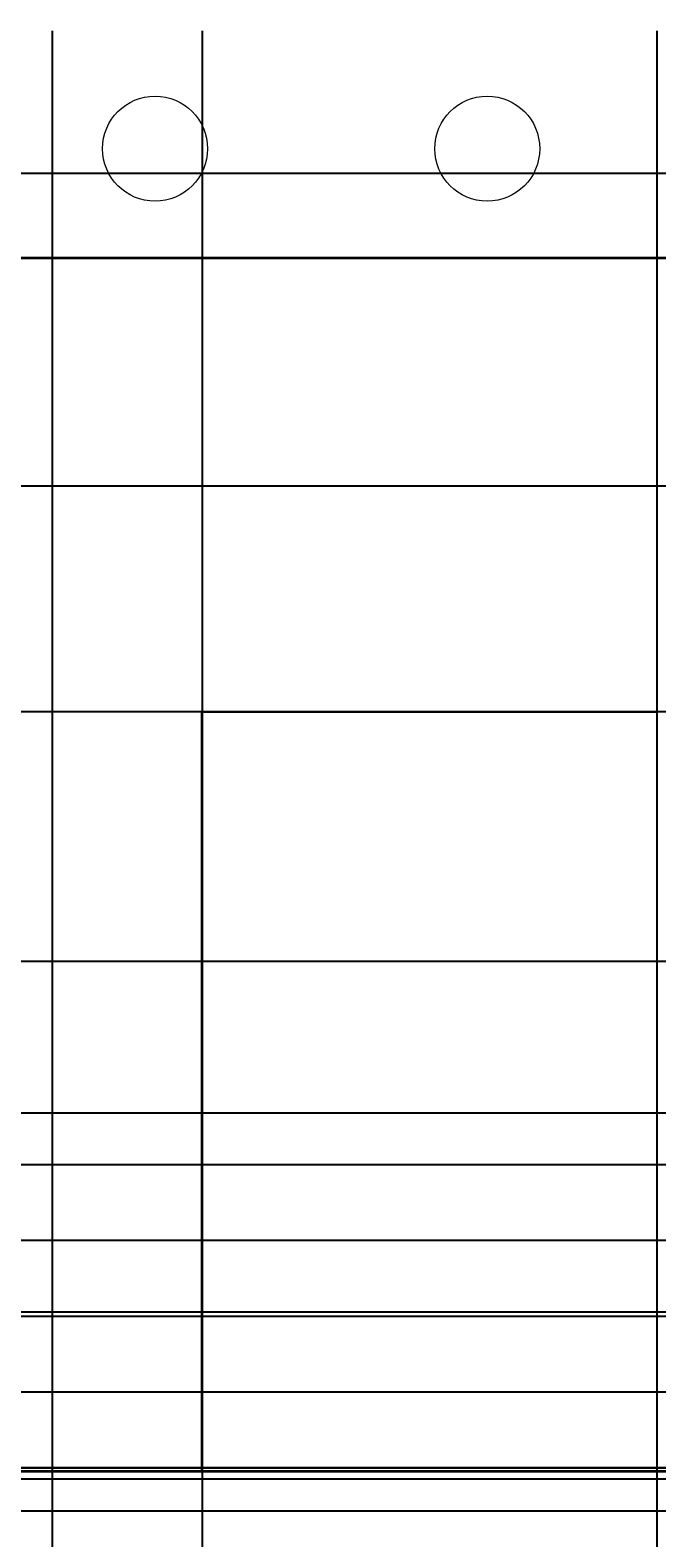
# Model space of a CAD drawing. Units: inches. Extents: x -13 to 809, y 112 to 656.
# Tile 9 of 55: x 111 to 161, y 205 to 325. Entities that reach past the tile are written whole.
import ezdxf

# ---------------------------------------------------------------- set-up
doc = ezdxf.new("R2010")
doc.units = ezdxf.units.IN
doc.header["$MEASUREMENT"] = 0
for name, color, linetype, lineweight in [('A-ANNO-DIMS', 2, 'Continuous', 18), ('A-DOOR', 4, 'Continuous', 25), ('A-ELEV', 7, 'Continuous', 35), ('A-ELEV-OTLN', 7, 'Continuous', 18)]:
    doc.layers.add(name, color=color, linetype=linetype, lineweight=lineweight)
doc.styles.get("Standard").update_dxf_attribs({"font": 'arial.ttf'})
doc.dimstyles.get("Standard").update_dxf_attribs({"dimtxt": 0.625, "dimasz": 0.18, "dimexe": 0.18, "dimexo": 0.0625, "dimgap": 0.09, "dimtad": 0, "dimtih": 1, "dimtoh": 1, "dimdec": 4, "dimzin": 0, "dimdsep": 46, "dimlunit": 4, "dimtxsty": 'Standard', "dimcen": 0.09, "dimadec": 0, "dimazin": 0, "dimtfac": 1, "dimtdec": 4, "dimtofl": 0, "dimtmove": 0, "dimatfit": 3, "dimfxl": 1, "dimtolj": 1, "dimtzin": 0, "dimarcsym": 0})

# ---------------------------------------------------------------- blocks, each defined once
blk = doc.blocks.new('*D12')
at = {"layer": 'A-ANNO-DIMS', "color": 0, "lineweight": -2, "transparency": 16777216}
for p, q in [((95.05, 306.46), (95.05, 112.34)), ((124.92, 210.46), (124.92, 112.34)), ((95.23, 112.52), (108.83, 112.52)), ((124.74, 112.52), (111.13, 112.52))]:
    blk.add_line(p, q, dxfattribs=at)
at = {"layer": 'A-ANNO-DIMS', "color": 0, "transparency": 16777216}
for points in [[(95.23, 112.55), (95.23, 112.49), (95.05, 112.52)], [(124.74, 112.55), (124.74, 112.49), (124.92, 112.52)]]:
    blk.add_solid(points, dxfattribs=at)
at = {"layer": 'Defpoints', "color": 0, "transparency": 16777216}
for p in [(95.05, 306.52), (124.92, 210.52), (124.92, 112.52)]:
    blk.add_point(p, dxfattribs=at)
at = {"layer": 'A-ANNO-DIMS', "color": 0, "transparency": 16777216, "insert": (109.98, 112.52), "char_height": 0.625, "attachment_point": 5}
blk.add_mtext('\\A1;29.87', dxfattribs=at)
blk = doc.blocks.new('*D13')
at = {"layer": 'A-ANNO-DIMS', "color": 0, "lineweight": -2, "transparency": 16777216}
for p, q in [((124.92, 210.46), (124.92, 112.34)), ((160.92, 210.46), (160.92, 112.34)), ((125.1, 112.52), (142.38, 112.52)), ((160.74, 112.52), (143.46, 112.52))]:
    blk.add_line(p, q, dxfattribs=at)
at = {"layer": 'A-ANNO-DIMS', "color": 0, "transparency": 16777216}
for points in [[(125.1, 112.55), (125.1, 112.49), (124.92, 112.52)], [(160.74, 112.55), (160.74, 112.49), (160.92, 112.52)]]:
    blk.add_solid(points, dxfattribs=at)
at = {"layer": 'Defpoints', "color": 0, "transparency": 16777216}
for p in [(124.92, 210.52), (160.92, 210.52), (160.92, 112.52)]:
    blk.add_point(p, dxfattribs=at)
at = {"layer": 'A-ANNO-DIMS', "color": 0, "transparency": 16777216, "insert": (142.92, 112.52), "char_height": 0.625, "attachment_point": 5}
blk.add_mtext('\\A1;36', dxfattribs=at)
blk = doc.blocks.new('*D39')
at = {"layer": 'A-ANNO-DIMS', "color": 0, "lineweight": -2, "transparency": 16777216}
for p, q in [((341.34, 524.28), (-12.1, 524.28)), ((-11.92, 524.1), (-11.92, 406.78)), ((-11.92, 288.63), (-11.92, 405.96)), ((341.34, 288.45), (-12.1, 288.45))]:
    blk.add_line(p, q, dxfattribs=at)
at = {"layer": 'A-ANNO-DIMS', "color": 0, "transparency": 16777216}
for points in [[(-11.95, 524.1), (-11.89, 524.1), (-11.92, 524.28)], [(-11.95, 288.63), (-11.89, 288.63), (-11.92, 288.45)]]:
    blk.add_solid(points, dxfattribs=at)
at = {"layer": 'Defpoints', "color": 0, "transparency": 16777216}
for p in [(-11.92, 524.28), (341.41, 524.28), (341.41, 288.45)]:
    blk.add_point(p, dxfattribs=at)
at = {"layer": 'A-ANNO-DIMS', "color": 0, "transparency": 16777216, "insert": (-11.92, 406.37), "char_height": 0.625, "attachment_point": 5}
blk.add_mtext('\\A1;235.83', dxfattribs=at)
blk = doc.blocks.new('*D40')
at = {"layer": 'A-ANNO-DIMS', "color": 0, "lineweight": -2, "transparency": 16777216}
for p, q in [((471.04, 313.17), (-12.1, 313.17)), ((-11.92, 312.99), (-11.92, 301.22)), ((-11.92, 288.63), (-11.92, 300.4)), ((341.34, 288.45), (-12.1, 288.45))]:
    blk.add_line(p, q, dxfattribs=at)
at = {"layer": 'A-ANNO-DIMS', "color": 0, "transparency": 16777216}
for points in [[(-11.95, 312.99), (-11.89, 312.99), (-11.92, 313.17)], [(-11.95, 288.63), (-11.89, 288.63), (-11.92, 288.45)]]:
    blk.add_solid(points, dxfattribs=at)
at = {"layer": 'Defpoints', "color": 0, "transparency": 16777216}
for p in [(471.1, 313.17), (-11.92, 288.45), (341.41, 288.45)]:
    blk.add_point(p, dxfattribs=at)
at = {"layer": 'A-ANNO-DIMS', "color": 0, "transparency": 16777216, "insert": (-11.92, 300.81), "char_height": 0.625, "attachment_point": 5}
blk.add_mtext('\\A1;24.716', dxfattribs=at)
blk = doc.blocks.new('*D41')
at = {"layer": 'A-ANNO-DIMS', "color": 0, "lineweight": -2, "transparency": 16777216}
for p, q in [((471.04, 357.98), (-12.1, 357.98)), ((-11.92, 357.8), (-11.92, 335.98)), ((-11.92, 313.35), (-11.92, 335.16)), ((471.04, 313.17), (-12.1, 313.17))]:
    blk.add_line(p, q, dxfattribs=at)
at = {"layer": 'A-ANNO-DIMS', "color": 0, "transparency": 16777216}
for points in [[(-11.95, 357.8), (-11.89, 357.8), (-11.92, 357.98)], [(-11.95, 313.35), (-11.89, 313.35), (-11.92, 313.17)]]:
    blk.add_solid(points, dxfattribs=at)
at = {"layer": 'Defpoints', "color": 0, "transparency": 16777216}
for p in [(-11.92, 357.98), (471.1, 357.98), (471.1, 313.17)]:
    blk.add_point(p, dxfattribs=at)
at = {"layer": 'A-ANNO-DIMS', "color": 0, "transparency": 16777216, "insert": (-11.92, 335.57), "char_height": 0.625, "attachment_point": 5}
blk.add_mtext('\\A1;44.81', dxfattribs=at)
blk = doc.blocks.new('*D44')
at = {"layer": 'A-ANNO-DIMS', "color": 0, "lineweight": -2, "transparency": 16777216}
for p, q in [((124.86, 270.6), (-12.1, 270.6)), ((-11.92, 270.42), (-11.92, 240.97)), ((-11.92, 210.7), (-11.92, 240.15)), ((124.86, 210.52), (-12.1, 210.52))]:
    blk.add_line(p, q, dxfattribs=at)
at = {"layer": 'A-ANNO-DIMS', "color": 0, "transparency": 16777216}
for points in [[(-11.95, 270.42), (-11.89, 270.42), (-11.92, 270.6)], [(-11.95, 210.7), (-11.89, 210.7), (-11.92, 210.52)]]:
    blk.add_solid(points, dxfattribs=at)
at = {"layer": 'Defpoints', "color": 0, "transparency": 16777216}
for p in [(-11.92, 270.6), (124.92, 270.6), (124.92, 210.52)]:
    blk.add_point(p, dxfattribs=at)
at = {"layer": 'A-ANNO-DIMS', "color": 0, "transparency": 16777216, "insert": (-11.92, 240.56), "char_height": 0.625, "attachment_point": 5}
blk.add_mtext('\\A1;60.08', dxfattribs=at)
blk = doc.blocks.new('*D45')
at = {"layer": 'A-ANNO-DIMS', "color": 0, "lineweight": -2, "transparency": 16777216}
for p, q in [((275.65, 270.6), (-12.1, 270.6)), ((-11.92, 270.42), (-11.92, 247.26)), ((-11.92, 223.28), (-11.92, 246.44)), ((275.65, 223.1), (-12.1, 223.1))]:
    blk.add_line(p, q, dxfattribs=at)
at = {"layer": 'A-ANNO-DIMS', "color": 0, "transparency": 16777216}
for points in [[(-11.95, 270.42), (-11.89, 270.42), (-11.92, 270.6)], [(-11.95, 223.28), (-11.89, 223.28), (-11.92, 223.1)]]:
    blk.add_solid(points, dxfattribs=at)
at = {"layer": 'Defpoints', "color": 0, "transparency": 16777216}
for p in [(-11.92, 270.6), (275.71, 270.6), (275.71, 223.1)]:
    blk.add_point(p, dxfattribs=at)
at = {"layer": 'A-ANNO-DIMS', "color": 0, "transparency": 16777216, "insert": (-11.92, 246.85), "char_height": 0.625, "attachment_point": 5}
blk.add_mtext('\\A1;47.5', dxfattribs=at)
blk = doc.blocks.new('*D49')
at = {"layer": 'A-ANNO-DIMS', "color": 0, "lineweight": -2, "transparency": 16777216}
for p, q in [((590.95, 250.84), (-12.1, 250.84)), ((-11.92, 250.66), (-11.92, 245.25)), ((-11.92, 239.02), (-11.92, 244.44)), ((590.95, 238.84), (-12.1, 238.84))]:
    blk.add_line(p, q, dxfattribs=at)
at = {"layer": 'A-ANNO-DIMS', "color": 0, "transparency": 16777216}
for points in [[(-11.95, 250.66), (-11.89, 250.66), (-11.92, 250.84)], [(-11.95, 239.02), (-11.89, 239.02), (-11.92, 238.84)]]:
    blk.add_solid(points, dxfattribs=at)
at = {"layer": 'Defpoints', "color": 0, "transparency": 16777216}
for p in [(-11.92, 250.84), (591.01, 250.84), (591.01, 238.84)]:
    blk.add_point(p, dxfattribs=at)
at = {"layer": 'A-ANNO-DIMS', "color": 0, "transparency": 16777216, "insert": (-11.92, 244.84), "char_height": 0.625, "attachment_point": 5}
blk.add_mtext('\\A1;12', dxfattribs=at)
blk = doc.blocks.new('*D50')
at = {"layer": 'A-ANNO-DIMS', "color": 0, "lineweight": -2, "transparency": 16777216}
for p, q in [((590.95, 238.84), (-12.1, 238.84)), ((-11.92, 238.66), (-11.92, 224.77)), ((-11.92, 210.06), (-11.92, 223.95)), ((607.51, 209.88), (-12.1, 209.88))]:
    blk.add_line(p, q, dxfattribs=at)
at = {"layer": 'A-ANNO-DIMS', "color": 0, "transparency": 16777216}
for points in [[(-11.95, 238.66), (-11.89, 238.66), (-11.92, 238.84)], [(-11.95, 210.06), (-11.89, 210.06), (-11.92, 209.88)]]:
    blk.add_solid(points, dxfattribs=at)
at = {"layer": 'Defpoints', "color": 0, "transparency": 16777216}
for p in [(591.01, 238.84), (-11.92, 209.88), (607.57, 209.88)]:
    blk.add_point(p, dxfattribs=at)
at = {"layer": 'A-ANNO-DIMS', "color": 0, "transparency": 16777216, "insert": (-11.92, 224.36), "char_height": 0.625, "attachment_point": 5}
blk.add_mtext('\\A1;28.97', dxfattribs=at)
blk = doc.blocks.new('*D80')
at = {"layer": 'A-ANNO-DIMS', "color": 0, "lineweight": -2, "transparency": 16777216}
for p, q in [((368.83, 216.77), (-12.1, 216.77)), ((-11.92, 216.59), (-11.92, 214.18)), ((-11.92, 210.95), (-11.92, 213.36)), ((368.83, 210.77), (-12.1, 210.77))]:
    blk.add_line(p, q, dxfattribs=at)
at = {"layer": 'A-ANNO-DIMS', "color": 0, "transparency": 16777216}
for points in [[(-11.95, 216.59), (-11.89, 216.59), (-11.92, 216.77)], [(-11.95, 210.95), (-11.89, 210.95), (-11.92, 210.77)]]:
    blk.add_solid(points, dxfattribs=at)
at = {"layer": 'Defpoints', "color": 0, "transparency": 16777216}
for p in [(-11.92, 216.77), (368.9, 216.77), (368.9, 210.77)]:
    blk.add_point(p, dxfattribs=at)
at = {"layer": 'A-ANNO-DIMS', "color": 0, "transparency": 16777216, "insert": (-11.92, 213.77), "char_height": 0.625, "attachment_point": 5}
blk.add_mtext('\\A1;6', dxfattribs=at)
blk = doc.blocks.new('*D81')
at = {"layer": 'A-ANNO-DIMS', "color": 0, "lineweight": -2, "transparency": 16777216}
for p, q in [((378.83, 222.77), (-12.1, 222.77)), ((-11.92, 222.59), (-11.92, 220.18)), ((-11.92, 216.95), (-11.92, 219.36)), ((378.83, 216.77), (-12.1, 216.77))]:
    blk.add_line(p, q, dxfattribs=at)
at = {"layer": 'A-ANNO-DIMS', "color": 0, "transparency": 16777216}
for points in [[(-11.95, 222.59), (-11.89, 222.59), (-11.92, 222.77)], [(-11.95, 216.95), (-11.89, 216.95), (-11.92, 216.77)]]:
    blk.add_solid(points, dxfattribs=at)
at = {"layer": 'Defpoints', "color": 0, "transparency": 16777216}
for p in [(-11.92, 222.77), (378.9, 222.77), (378.9, 216.77)]:
    blk.add_point(p, dxfattribs=at)
at = {"layer": 'A-ANNO-DIMS', "color": 0, "transparency": 16777216, "insert": (-11.92, 219.77), "char_height": 0.625, "attachment_point": 5}
blk.add_mtext('\\A1;6', dxfattribs=at)
blk = doc.blocks.new('*D82')
at = {"layer": 'A-ANNO-DIMS', "color": 0, "lineweight": -2, "transparency": 16777216}
for p, q in [((388.83, 228.77), (-12.1, 228.77)), ((-11.92, 228.59), (-11.92, 226.18)), ((-11.92, 222.95), (-11.92, 225.36)), ((388.83, 222.77), (-12.1, 222.77))]:
    blk.add_line(p, q, dxfattribs=at)
at = {"layer": 'A-ANNO-DIMS', "color": 0, "transparency": 16777216}
for points in [[(-11.95, 228.59), (-11.89, 228.59), (-11.92, 228.77)], [(-11.95, 222.95), (-11.89, 222.95), (-11.92, 222.77)]]:
    blk.add_solid(points, dxfattribs=at)
at = {"layer": 'Defpoints', "color": 0, "transparency": 16777216}
for p in [(-11.92, 228.77), (388.9, 228.77), (388.9, 222.77)]:
    blk.add_point(p, dxfattribs=at)
at = {"layer": 'A-ANNO-DIMS', "color": 0, "transparency": 16777216, "insert": (-11.92, 225.77), "char_height": 0.625, "attachment_point": 5}
blk.add_mtext('\\A1;6', dxfattribs=at)
blk = doc.blocks.new('*D83')
at = {"layer": 'A-ANNO-DIMS', "color": 0, "lineweight": -2, "transparency": 16777216}
for p, q in [((398.83, 234.77), (-12.1, 234.77)), ((-11.92, 234.59), (-11.92, 232.18)), ((-11.92, 228.95), (-11.92, 231.36)), ((398.83, 228.77), (-12.1, 228.77))]:
    blk.add_line(p, q, dxfattribs=at)
at = {"layer": 'A-ANNO-DIMS', "color": 0, "transparency": 16777216}
for points in [[(-11.95, 234.59), (-11.89, 234.59), (-11.92, 234.77)], [(-11.95, 228.95), (-11.89, 228.95), (-11.92, 228.77)]]:
    blk.add_solid(points, dxfattribs=at)
at = {"layer": 'Defpoints', "color": 0, "transparency": 16777216}
for p in [(-11.92, 234.77), (398.9, 234.77), (398.9, 228.77)]:
    blk.add_point(p, dxfattribs=at)
at = {"layer": 'A-ANNO-DIMS', "color": 0, "transparency": 16777216, "insert": (-11.92, 231.77), "char_height": 0.625, "attachment_point": 5}
blk.add_mtext('\\A1;6', dxfattribs=at)
blk = doc.blocks.new('*D84')
at = {"layer": 'A-ANNO-DIMS', "color": 0, "lineweight": -2, "transparency": 16777216}
for p, q in [((408.83, 238.84), (-12.1, 238.84)), ((-11.92, 238.66), (-11.92, 237.22)), ((-11.92, 234.95), (-11.92, 236.4)), ((408.83, 234.77), (-12.1, 234.77))]:
    blk.add_line(p, q, dxfattribs=at)
at = {"layer": 'A-ANNO-DIMS', "color": 0, "transparency": 16777216}
for points in [[(-11.95, 238.66), (-11.89, 238.66), (-11.92, 238.84)], [(-11.95, 234.95), (-11.89, 234.95), (-11.92, 234.77)]]:
    blk.add_solid(points, dxfattribs=at)
at = {"layer": 'Defpoints', "color": 0, "transparency": 16777216}
for p in [(-11.92, 238.84), (408.9, 238.84), (408.9, 234.77)]:
    blk.add_point(p, dxfattribs=at)
at = {"layer": 'A-ANNO-DIMS', "color": 0, "transparency": 16777216, "insert": (-11.92, 236.81), "char_height": 0.625, "attachment_point": 5}
blk.add_mtext('\\A1;4.069', dxfattribs=at)
blk = doc.blocks.new('*D94')
at = {"layer": 'A-ANNO-DIMS', "color": 0, "lineweight": -2, "transparency": 16777216}
for p, q in [((210.02, 223.1), (-12.1, 223.1)), ((-11.92, 222.92), (-11.92, 217.22)), ((-11.92, 210.7), (-11.92, 216.4)), ((160.86, 210.52), (-12.1, 210.52))]:
    blk.add_line(p, q, dxfattribs=at)
at = {"layer": 'A-ANNO-DIMS', "color": 0, "transparency": 16777216}
for points in [[(-11.95, 222.92), (-11.89, 222.92), (-11.92, 223.1)], [(-11.95, 210.7), (-11.89, 210.7), (-11.92, 210.52)]]:
    blk.add_solid(points, dxfattribs=at)
at = {"layer": 'Defpoints', "color": 0, "transparency": 16777216}
for p in [(-11.92, 223.1), (210.08, 223.1), (160.92, 210.52)]:
    blk.add_point(p, dxfattribs=at)
at = {"layer": 'A-ANNO-DIMS', "color": 0, "transparency": 16777216, "insert": (-11.92, 216.81), "char_height": 0.625, "attachment_point": 5}
blk.add_mtext('\\A1;12.58', dxfattribs=at)
blk = doc.blocks.new('*D107')
at = {"layer": 'A-ANNO-DIMS', "color": 0, "lineweight": -2, "transparency": 16777216}
for p, q in [((113.05, 324.46), (113.05, 112.34)), ((95.05, 306.46), (95.05, 112.34)), ((95.23, 112.52), (102.93, 112.52)), ((112.87, 112.52), (105.16, 112.52))]:
    blk.add_line(p, q, dxfattribs=at)
at = {"layer": 'A-ANNO-DIMS', "color": 0, "transparency": 16777216}
for points in [[(95.23, 112.55), (95.23, 112.49), (95.05, 112.52)], [(112.87, 112.55), (112.87, 112.49), (113.05, 112.52)]]:
    blk.add_solid(points, dxfattribs=at)
at = {"layer": 'Defpoints', "color": 0, "transparency": 16777216}
for p in [(113.05, 324.52), (95.05, 306.52), (113.05, 112.52)]:
    blk.add_point(p, dxfattribs=at)
at = {"layer": 'A-ANNO-DIMS', "color": 0, "transparency": 16777216, "insert": (104.05, 112.52), "char_height": 0.625, "attachment_point": 5}
blk.add_mtext('\\A1;18.00', dxfattribs=at)
blk = doc.blocks.new('*D109')
at = {"layer": 'A-ANNO-DIMS', "color": 0, "lineweight": -2, "transparency": 16777216}
for p, q in [((113.05, 324.46), (113.05, 112.34)), ((124.92, 324.46), (124.92, 112.34)), ((113.23, 112.52), (117.63, 112.52)), ((124.74, 112.52), (120.34, 112.52))]:
    blk.add_line(p, q, dxfattribs=at)
at = {"layer": 'A-ANNO-DIMS', "color": 0, "transparency": 16777216}
for points in [[(113.23, 112.55), (113.23, 112.49), (113.05, 112.52)], [(124.74, 112.55), (124.74, 112.49), (124.92, 112.52)]]:
    blk.add_solid(points, dxfattribs=at)
at = {"layer": 'Defpoints', "color": 0, "transparency": 16777216}
for p in [(113.05, 324.52), (124.92, 324.52), (124.92, 112.52)]:
    blk.add_point(p, dxfattribs=at)
at = {"layer": 'A-ANNO-DIMS', "color": 0, "transparency": 16777216, "insert": (118.98, 112.52), "char_height": 0.625, "attachment_point": 5}
blk.add_mtext('\\A1;11.872', dxfattribs=at)
blk = doc.blocks.new('*D110')
at = {"layer": 'A-ANNO-DIMS', "color": 0, "lineweight": -2, "transparency": 16777216}
for p, q in [((124.92, 324.46), (124.92, 112.34)), ((160.92, 324.46), (160.92, 112.34)), ((125.1, 112.52), (141.78, 112.52)), ((160.74, 112.52), (144.06, 112.52))]:
    blk.add_line(p, q, dxfattribs=at)
at = {"layer": 'A-ANNO-DIMS', "color": 0, "transparency": 16777216}
for points in [[(125.1, 112.55), (125.1, 112.49), (124.92, 112.52)], [(160.74, 112.55), (160.74, 112.49), (160.92, 112.52)]]:
    blk.add_solid(points, dxfattribs=at)
at = {"layer": 'Defpoints', "color": 0, "transparency": 16777216}
for p in [(124.92, 324.52), (160.92, 324.52), (160.92, 112.52)]:
    blk.add_point(p, dxfattribs=at)
at = {"layer": 'A-ANNO-DIMS', "color": 0, "transparency": 16777216, "insert": (142.92, 112.52), "char_height": 0.625, "attachment_point": 5}
blk.add_mtext('\\A1;36.00', dxfattribs=at)
blk = doc.blocks.new('*D115')
at = {"layer": 'A-ANNO-DIMS', "color": 0, "lineweight": -2, "transparency": 16777216}
for p, q in [((311.4, 210.78), (-12.1, 210.78)), ((-11.92, 210.6), (-11.92, 181.06)), ((-11.92, 150.7), (-11.92, 180.24)), ((311.64, 150.52), (-12.1, 150.52))]:
    blk.add_line(p, q, dxfattribs=at)
at = {"layer": 'A-ANNO-DIMS', "color": 0, "transparency": 16777216}
for points in [[(-11.95, 210.6), (-11.89, 210.6), (-11.92, 210.78)], [(-11.95, 150.7), (-11.89, 150.7), (-11.92, 150.52)]]:
    blk.add_solid(points, dxfattribs=at)
at = {"layer": 'Defpoints', "color": 0, "transparency": 16777216}
for p in [(-11.92, 210.78), (311.46, 210.78), (311.7, 150.52)]:
    blk.add_point(p, dxfattribs=at)
at = {"layer": 'A-ANNO-DIMS', "color": 0, "transparency": 16777216, "insert": (-11.92, 180.65), "char_height": 0.625, "attachment_point": 5}
blk.add_mtext('\\A1;60.27', dxfattribs=at)
blk = doc.blocks.new('*D118')
at = {"layer": 'A-ANNO-DIMS', "color": 0, "lineweight": -2, "transparency": 16777216}
for p, q in [((311.4, 210.78), (-12.1, 210.78)), ((-11.92, 210.6), (-11.92, 209.49)), ((-11.92, 207.55), (-11.92, 208.67)), ((308.59, 207.37), (-12.1, 207.37))]:
    blk.add_line(p, q, dxfattribs=at)
at = {"layer": 'A-ANNO-DIMS', "color": 0, "transparency": 16777216}
for points in [[(-11.95, 210.6), (-11.89, 210.6), (-11.92, 210.78)], [(-11.95, 207.55), (-11.89, 207.55), (-11.92, 207.37)]]:
    blk.add_solid(points, dxfattribs=at)
at = {"layer": 'Defpoints', "color": 0, "transparency": 16777216}
for p in [(-11.92, 210.78), (311.46, 210.78), (308.65, 207.37)]:
    blk.add_point(p, dxfattribs=at)
at = {"layer": 'A-ANNO-DIMS', "color": 0, "transparency": 16777216, "insert": (-11.92, 209.08), "char_height": 0.625, "attachment_point": 5}
blk.add_mtext('\\A1;3.41', dxfattribs=at)

msp = doc.modelspace()

# ---------------------------------------------------------------- linework, layer by layer
at = {"layer": 'A-DOOR'}
for p, q in [((124.9184, 210.5199), (124.9184, 270.6024)), ((124.9184, 270.6024), (160.9184, 270.6024)), ((160.9184, 270.6024), (160.9184, 210.5199))]:
    msp.add_line(p, q, dxfattribs=at)
at = {"layer": 'A-ELEV'}
for p, q in [((109.5888, 306.5199), (337.5074, 306.5199)), ((26.0809, 210.5199), (256.4464, 210.5199))]:
    msp.add_line(p, q, dxfattribs=at)
at = {"layer": 'A-ELEV-OTLN'}
for centre in [(121.2048, 315.1435), (147.4935, 315.1435)]:
    msp.add_circle(centre, 4.1542, dxfattribs=at)

# ---------------------------------------------------------------- dimensions: what is measured, and where the dimension line sits
at = {"layer": 'A-ANNO-DIMS'}
for base, p1, p2, override, picture, middle in [((-11.9191, 524.281), (341.4072, 288.4508), (341.4072, 524.281), {"dimdec": 2, "dimlfac": 1, "dimrnd": 0, "dimzin": 0, "dimdsep": 46, "dimlunit": 2}, '*D39', (-11.9191, 406.3659)), ((-11.9191, 357.9804), (471.0998, 313.1667), (471.0998, 357.9804), {"dimdec": 2, "dimlfac": 1, "dimrnd": 0, "dimzin": 0, "dimdsep": 46, "dimlunit": 2}, '*D41', (-11.9191, 335.5735)), ((-11.9191, 288.4508), (471.0998, 313.1667), (341.4072, 288.4508), {"dimdec": 3, "dimlfac": 1, "dimrnd": 0, "dimzin": 0, "dimdsep": 46, "dimlunit": 2}, '*D40', (-11.9191, 300.8087)), ((-11.9191, 270.6024), (124.9184, 210.5199), (124.9184, 270.6024), {"dimdec": 2, "dimlfac": 1, "dimrnd": 0, "dimzin": 0, "dimdsep": 46, "dimlunit": 2}, '*D44', (-11.9191, 240.5611)), ((-11.9191, 270.6024), (275.7145, 223.1), (275.7145, 270.6024), {"dimdec": 1, "dimlfac": 1, "dimrnd": 0, "dimzin": 0, "dimdsep": 46, "dimlunit": 2}, '*D45', (-11.9191, 246.8512)), ((-11.9191, 250.8429), (591.008, 238.8429), (591.008, 250.8429), {"dimdec": 0, "dimlfac": 1, "dimrnd": 0, "dimzin": 0, "dimdsep": 46, "dimlunit": 2}, '*D49', (-11.9191, 244.8429)), ((-11.9191, 209.8753), (591.008, 238.8429), (607.5741, 209.8753), {"dimdec": 2, "dimlfac": 1, "dimrnd": 0, "dimzin": 0, "dimdsep": 46, "dimlunit": 2}, '*D50', (-11.9191, 224.3591)), ((-11.9191, 238.8429), (408.8966, 234.7738), (408.8966, 238.8429), {"dimdec": 3, "dimlfac": 1, "dimrnd": 0, "dimzin": 0, "dimdsep": 46, "dimlunit": 2}, '*D84', (-11.9191, 236.8083)), ((-11.9191, 234.7738), (398.8966, 228.7738), (398.8966, 234.7738), {"dimdec": 0, "dimlfac": 1, "dimrnd": 0, "dimzin": 0, "dimdsep": 46, "dimlunit": 2}, '*D83', (-11.9191, 231.7738)), ((-11.9191, 228.7738), (388.8966, 222.7738), (388.8966, 228.7738), {"dimdec": 0, "dimlfac": 1, "dimrnd": 0, "dimzin": 0, "dimdsep": 46, "dimlunit": 2}, '*D82', (-11.9191, 225.7738)), ((-11.9191, 223.1), (160.9184, 210.5199), (210.0791, 223.1), {"dimdec": 2, "dimlfac": 1, "dimrnd": 0, "dimzin": 0, "dimdsep": 46, "dimlunit": 2}, '*D94', (-11.9191, 216.81)), ((-11.9191, 222.7738), (378.8966, 216.7738), (378.8966, 222.7738), {"dimdec": 0, "dimlfac": 1, "dimrnd": 0, "dimzin": 0, "dimdsep": 46, "dimlunit": 2}, '*D81', (-11.9191, 219.7738)), ((-11.9191, 216.7738), (368.8966, 210.7738), (368.8966, 216.7738), {"dimdec": 0, "dimlfac": 1, "dimrnd": 0, "dimzin": 0, "dimdsep": 46, "dimlunit": 2}, '*D80', (-11.9191, 213.7738)), ((-11.91915, 210.78493), (311.6991, 150.51989), (311.46269, 210.78493), {"dimdec": 2, "dimlfac": 1, "dimrnd": 0, "dimzin": 0, "dimdsep": 46, "dimlunit": 2}, '*D115', (-11.91915, 180.65241)), ((-11.9191, 210.7849), (308.6488, 207.3724), (311.4627, 210.7849), {"dimdec": 2, "dimlfac": 1, "dimrnd": 0, "dimzin": 0, "dimdsep": 46, "dimlunit": 2}, '*D118', (-11.9191, 209.0787))]:
    dim = msp.add_linear_dim(base=base, p1=p1, p2=p2, angle=90, dimstyle='Standard', override=override, dxfattribs=at)
    dim.commit()
    dim.dimension.update_dxf_attribs({"geometry": picture, "text_midpoint": middle})
for base, p1, p2, override, picture, middle in [((113.0469, 112.5199), (95.0469, 306.5199), (113.0469, 324.5199), {"dimdec": 2, "dimlfac": 1, "dimrnd": 0, "dimzin": 0, "dimdsep": 46, "dimlunit": 2}, '*D107', (104.0469, 112.5199)), ((124.91845, 112.51989), (113.04686, 324.51989), (124.91845, 324.51989), {"dimdec": 3, "dimlfac": 1, "dimrnd": 0, "dimzin": 0, "dimdsep": 46, "dimlunit": 2}, '*D109', (118.98265, 112.51989)), ((160.9184, 112.5199), (124.9184, 324.5199), (160.9184, 324.5199), {"dimdec": 2, "dimlfac": 1, "dimrnd": 0, "dimzin": 0, "dimdsep": 46, "dimlunit": 2}, '*D110', (142.9184, 112.5199)), ((124.9184, 112.5199), (95.0469, 306.5199), (124.9184, 210.5199), {"dimdec": 2, "dimlfac": 1, "dimrnd": 0, "dimzin": 0, "dimdsep": 46, "dimlunit": 2}, '*D12', (109.9827, 112.5199)), ((160.9184, 112.5199), (124.9184, 210.5199), (160.9184, 210.5199), {"dimdec": 0, "dimlfac": 1, "dimrnd": 0, "dimzin": 0, "dimdsep": 46, "dimlunit": 2}, '*D13', (142.9184, 112.5199))]:
    dim = msp.add_linear_dim(base=base, p1=p1, p2=p2, dimstyle='Standard', override=override, dxfattribs=at)
    dim.commit()
    dim.dimension.update_dxf_attribs({"geometry": picture, "text_midpoint": middle})

doc.saveas('drawing.dxf')
